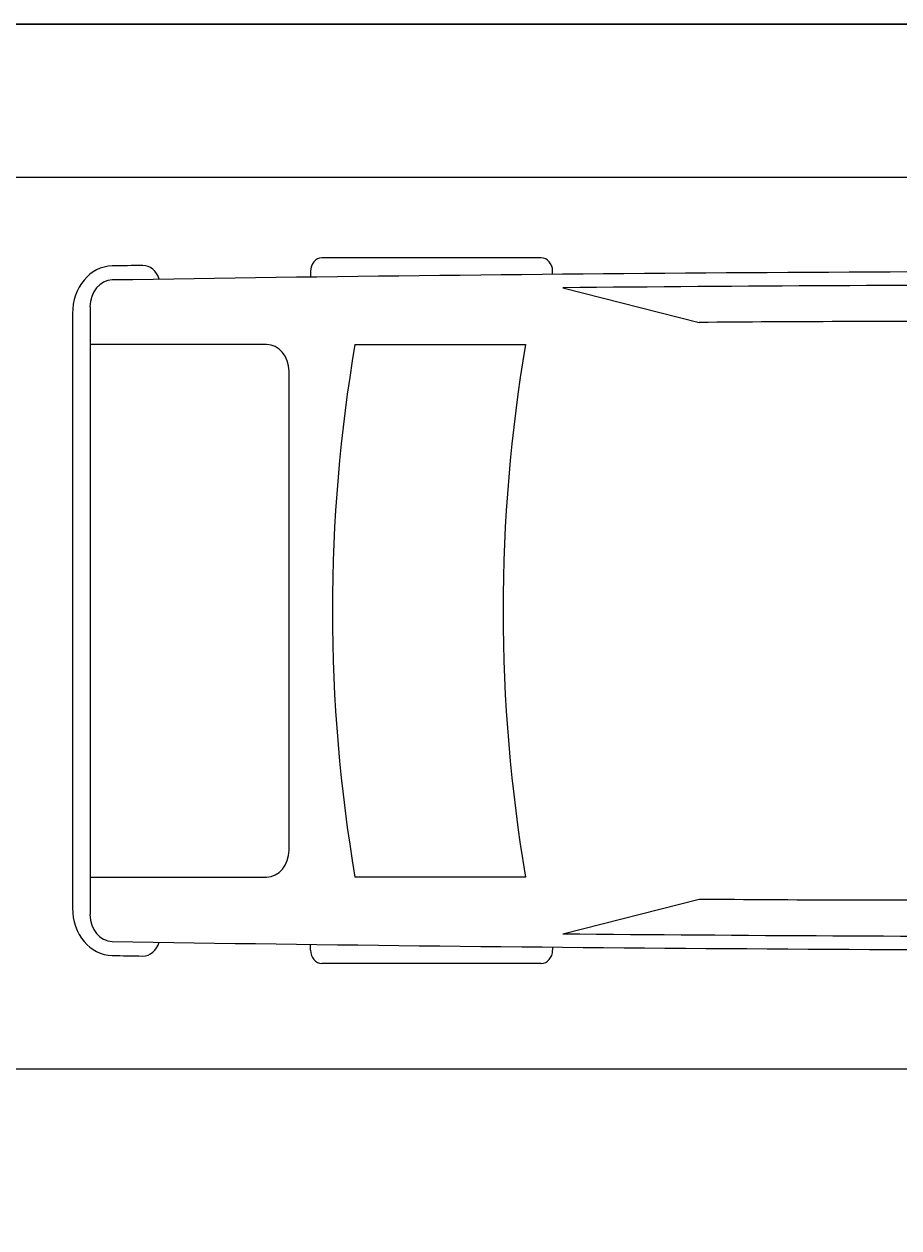
# Model space of a CAD drawing. Units: inches. Extents: x -46 to 1145, y -527 to 760.
# Tile 11 of 57: x 283 to 380, y -172 to -39. Entities that reach past the tile are written whole.
import ezdxf

# ---------------------------------------------------------------- set-up
doc = ezdxf.new("R2010")
doc.units = ezdxf.units.IN
doc.header["$MEASUREMENT"] = 0
for name, color, linetype, lineweight in [('A-ANNO-DIMS', 2, 'Continuous', 18), ('C-PKNG', 8, 'Continuous', 18), ('C-PKNG-VEHI', 8, 'Continuous', 13), ('C-SITE', 7, 'Continuous', 30)]:
    doc.layers.add(name, color=color, linetype=linetype, lineweight=lineweight)
doc.styles.get("Standard").update_dxf_attribs({"font": 'arial.ttf'})
doc.dimstyles.get("Standard").update_dxf_attribs({"dimtxt": 0.18, "dimasz": 0.18, "dimexe": 0.18, "dimexo": 0.0625, "dimgap": 0.09, "dimtad": 0, "dimtih": 1, "dimtoh": 1, "dimdec": 0, "dimzin": 0, "dimdsep": 46, "dimlunit": 3, "dimtxsty": 'Standard', "dimcen": 0.09, "dimadec": 0, "dimazin": 0, "dimtfac": 1, "dimtdec": 0, "dimtofl": 0, "dimtmove": 0, "dimatfit": 3, "dimfxl": 1, "dimtolj": 1, "dimtzin": 0, "dimarcsym": 0})

# ---------------------------------------------------------------- blocks, each defined once
blk = doc.blocks.new('*U640')
for p, q in [((1182.5, 987.8), (567.7, 987.8)), ((3472.1, 987.8), (4086.9, 987.8)), ((536, 950.2), (536, 935.5)), ((1214.1, 949.7), (1214.1, 950.2)), ((3440.5, 941.7), (3440.5, 950.2)), ((4118.5, 950.2), (4118.5, 934.1)), ((2234.8, 809.5), (1898.9, 912.4)), ((3411.6, 904.3), (3029.9, 807.2)), ((4736.4, -850.9), (4736.4, 850.9)), ((4785.3, -832.1), (4785.3, 832.1)), ((1778.8, 801), (2194.7, 745.5)), ((3515.9, 745.5), (3994.1, 745.5)), ((4736.4, 745.5), (4242, 745.5)), ((4178.7, 670.3), (4178.7, -670.3)), ((819.6, 295.3), (917.7, 436.1)), ((917.7, 436.1), (1293.8, 436.1)), ((815.9, 241.4), (815.9, 283.3)), ((1496.5, -273.7), (1496.5, 273.7)), ((756.2, 241.4), (1312.8, 241.4)), ((1690.4, -267.4), (1690.4, 267.4)), ((4736.4, -267.4), (4736.4, 267.4)), ((2101.5, 215.8), (2101.5, -215.8)), ((83, 155.7), (2.6, 10.3)), ((0, 0), (1312.8, 0)), ((2.6, -10.3), (83, -155.7)), ((756.2, -241.4), (1312.8, -241.4)), ((815.9, -241.4), (815.9, -283.3)), ((819.6, -295.3), (917.7, -436.1)), ((917.7, -436.1), (1293.8, -436.1)), ((2194.7, -745.5), (1778.8, -801)), ((3994.1, -745.5), (3515.9, -745.5)), ((4242, -745.5), (4736.4, -745.5)), ((3411.6, -904.3), (3029.9, -807.2)), ((2234.8, -809.5), (1898.9, -912.4)), ((536, -950.2), (536, -935.5)), ((3440.5, -941.7), (3440.5, -950.2)), ((4118.5, -950.2), (4118.5, -934.1)), ((1214.1, -949.7), (1214.1, -950.2)), ((1182.5, -987.8), (567.7, -987.8)), ((3472.1, -987.8), (4086.9, -987.8))]:
    blk.add_line(p, q)
for centre, major_axis, ratio, start_param, end_param in [((567.7, 950.2), (0, -37.6), 0.842304, 3.141593, 4.712389), ((1182.5, 950.2), (0, 37.6), 0.842304, -1.570796, 0), ((3472.1, 950.2), (0, -37.6), 0.842304, 3.141593, 4.712389), ((4086.9, 950.2), (0, 37.6), 0.842304, -1.570796, 0), ((1046.3, -12467.9), (0, 13417.1), 0.842304, 0.00281, 0.075598), ((1637.8, -268112.7), (0, 269062.9), 0.842304, -0.013397, 0.002797), ((4588, 910.3), (0, 56.4), 0.842304, -0.013017, 1.249894), ((1637.8, -268131.5), (0, 269121), 0.842304, -0.013397, -0.013017), ((4673.1, 832.1), (0, -133.3), 0.842304, 1.570796, 3.128196), ((6757.2, -699.1), (0, 7958), 0.842304, 1.367076, 1.39176), ((1637.8, -268112.7), (0, -269025.3), 0.842304, 3.133765, 3.140441), ((4673.1, 850.9), (0, -75.2), 0.842304, 1.570796, 3.128196), ((2433, -93125.4), (0, -93935.2), 0.842304, 3.134049, 3.144098), ((3436.4, 136.8), (0, 2077), 0.842304, 1.245306, 1.50788), ((951.8, -15086.6), (0, -15832.5), 0.842304, 3.096046, 3.200911), ((3799.7, 71.1), (0, -2021.3), 0.842304, 4.372215, 4.640744), ((433.9, 0), (0, 3734.3), 0.842304, 4.511394, 4.913384), ((912, 0), (0, 3734.3), 0.842304, 4.511394, 4.913384), ((4242, 670.3), (0, 75.2), 0.842304, 0, 1.570796), ((6583, -699.1), (0, -7754.7), 0.842304, 4.528606, 4.561838), ((3413.8, 136.8), (0, -2280.3), 0.842304, 4.449482, 4.652344), ((-5194.2, 1330.9), (0, -6374.4), 0.842304, 1.385369, 1.434372), ((331.1, 432), (0, 696.4), 0.842304, 4.435146, 4.718221), ((360.7, 432), (0, 696.4), 0.842304, 4.435146, 4.718221), ((1290.1, 338.8), (161, -9.1), 0.603834, -1.395552, 1.581315), ((831.8, 283.3), (0, 18.8), 0.842304, 0.879714, 1.570796), ((756.2, -1185.2), (0, 1426.7), 0.842304, 0, 0.590319), ((15.8, 0), (0, -18.8), 0.842304, 4.131459, 5.293319), ((756.2, 1185.2), (0, 1426.7), 0.842304, 2.551274, 3.141593), ((-5194.2, -1330.9), (0, 6374.4), 0.842304, -1.434372, -1.385369), ((3799.7, -71.1), (0, -2021.3), 0.842304, -1.499151, -1.230623), ((331.1, -432), (0, -696.4), 0.842304, 1.564964, 1.848039), ((360.7, -432), (0, -696.4), 0.842304, 1.564964, 1.848039), ((3436.4, -136.8), (0, -2077), 0.842304, -1.50788, -1.245306), ((831.8, -283.3), (0, -18.8), 0.842304, 4.712389, 5.403472), ((3413.8, -136.8), (0, -2280.3), 0.842304, -1.510751, -1.307889), ((6583, 699.1), (0, 7754.7), 0.842304, 1.721348, 1.754579), ((4242, -670.3), (0, -75.2), 0.842304, 4.712389, 6.283185), ((6757.2, 699.1), (0, 7958), 0.842304, 1.749832, 1.774517), ((951.8, 15086.6), (0, -15832.5), 0.842304, -0.059319, 0.045547), ((2433, 93125.4), (0, -93935.2), 0.842304, -0.002505, 0.007544), ((4673.1, -832.1), (0, -133.3), 0.842304, 0.013397, 1.570796), ((4673.1, -850.9), (0, 75.2), 0.842304, 3.15499, 4.712389), ((1637.8, 268112.7), (0, -269025.3), 0.842304, 0.001152, 0.007828), ((1046.3, 12467.9), (0, -13417.1), 0.842304, -0.075598, -0.00281), ((1637.8, 268112.7), (0, 269062.9), 0.842304, 3.138796, 3.15499), ((4588, -910.3), (0, -56.4), 0.842304, -1.249894, 0.013017), ((567.7, -950.2), (0, 37.6), 0.842304, 1.570796, 3.141593), ((1182.5, -950.2), (0, -37.6), 0.842304, 0, 1.570796), ((3472.1, -950.2), (0, -37.6), 0.842304, -1.570796, 0), ((4086.9, -950.2), (0, 37.6), 0.842304, 3.141593, 4.712389), ((1637.8, 268131.5), (0, 269121), 0.842304, 3.15461, 3.15499)]:
    blk.add_ellipse(centre, major_axis=major_axis, ratio=ratio, start_param=start_param, end_param=end_param)
at = {"extrusion": (0, 0, -1)}
blk.add_ellipse((1290.1, -338.8), major_axis=(161, 9.1), ratio=0.603834, start_param=-1.395552, end_param=1.581315, dxfattribs=at)
blk = doc.blocks.new('*D702')
at = {"layer": 'A-ANNO-DIMS', "color": 0, "lineweight": -2, "transparency": 16777216}
for p, q in [((189.63, -39.48), (1145.34, -39.48)), ((1145.16, -39.66), (1145.16, -249.3)), ((1145.16, -459.3), (1145.16, -249.66)), ((183.63, -459.48), (1145.34, -459.48))]:
    blk.add_line(p, q, dxfattribs=at)
at = {"layer": 'A-ANNO-DIMS', "color": 0, "transparency": 16777216}
for points in [[(1145.13, -39.66), (1145.19, -39.66), (1145.16, -39.48)], [(1145.13, -459.3), (1145.19, -459.3), (1145.16, -459.48)]]:
    blk.add_solid(points, dxfattribs=at)
at = {"layer": 'Defpoints', "color": 0, "transparency": 16777216}
for p in [(189.56, -39.48), (1145.16, -39.48), (183.56, -459.48)]:
    blk.add_point(p, dxfattribs=at)
at = {"layer": 'A-ANNO-DIMS', "color": 0, "transparency": 16777216, "insert": (1145.16, -249.48), "char_height": 0.18, "attachment_point": 5}
blk.add_mtext('\\A1;420', dxfattribs=at)

msp = doc.modelspace()

# ---------------------------------------------------------------- linework, layer by layer
at = {"layer": 'C-PKNG'}
msp.add_lwpolyline([(501.7297, -154.6684), (273.5156, -154.6684), (273.5156, -56.3706), (501.7297, -56.3706)], close=True, dxfattribs=at)
at = {"layer": 'C-SITE'}
msp.add_line((590.0637, -39.4824), (189.5637, -39.4824), dxfattribs=at)

# ---------------------------------------------------------------- block references
at = {"layer": 'C-PKNG-VEHI', "xscale": 0.0393700787401575, "yscale": 0.0393700787401575, "zscale": 0.0393700787401575, "rotation": 180}
msp.add_blockref('*U640', (476.808, -104.1506), dxfattribs=at)

# ---------------------------------------------------------------- dimensions: what is measured, and where the dimension line sits
at = {"layer": 'A-ANNO-DIMS'}
dim = msp.add_linear_dim(base=(1145.1637, -39.4824), p1=(183.5637, -459.4824), p2=(189.5637, -39.4824), angle=90, dimstyle='Standard', override={"dimdec": 0, "dimlfac": 1, "dimrnd": 0, "dimzin": 0, "dimdsep": 46, "dimlunit": 2}, dxfattribs=at)
dim.commit()
dim.dimension.update_dxf_attribs({"geometry": '*D702', "text_midpoint": (1145.1637, -249.4824)})

doc.saveas('drawing.dxf')
